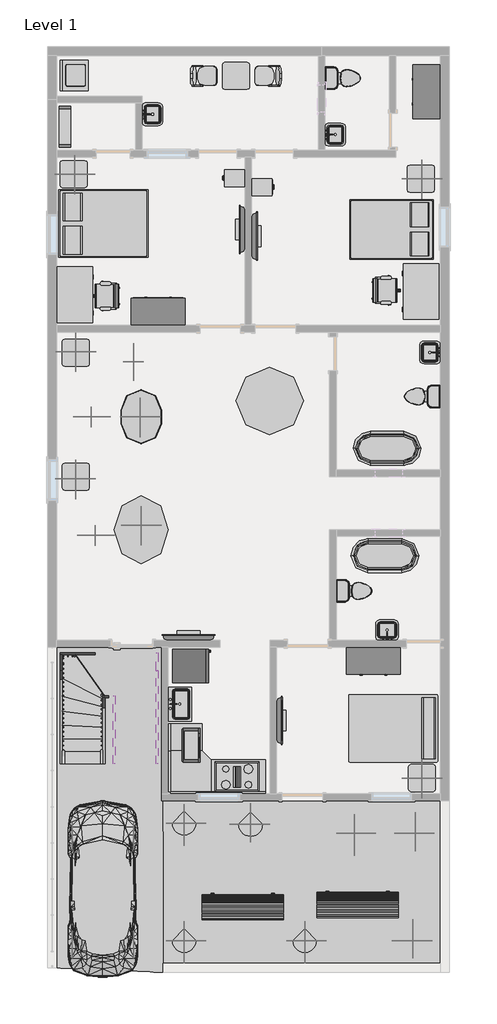
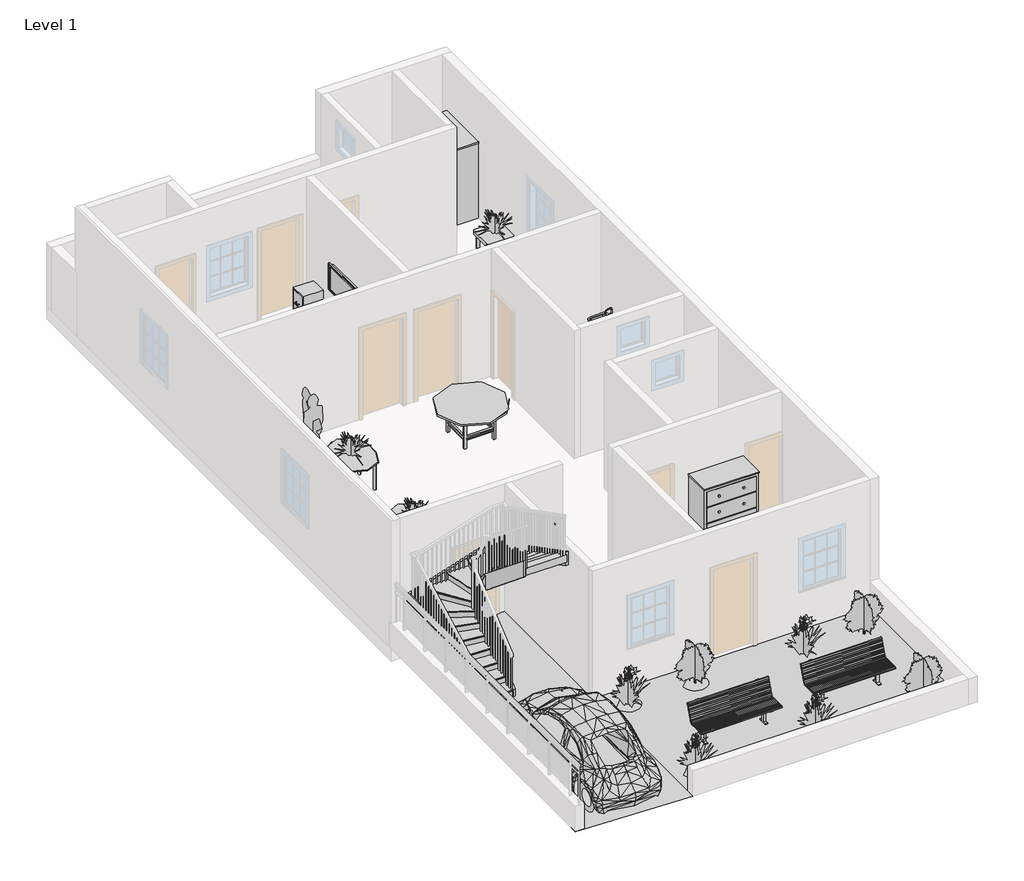
# One storey, part 3 of 3: 29 furniture elements, 16 geographic elements, 14 flow terminals, 10 proxies, 8 members, 1 stair flight.
"""IFC4 building model written with IfcOpenShell, lengths in millimetres."""

from ifc_helpers import new_model, si_unit, frame, origin, place, context, project, spatial, polyline, outline, extrude, triangles, transform, mapped, element, save
from components import proxy_bb1e6e30, proxy_8a8d5ab2, rpc_beetle_rpc_beetle_3ce7ba48, rpc_female_69e001fa, proxy_a13a33b2, proxy_718fa39f, flow_terminal_2b63360b, flow_terminal_accce45a, flow_terminal_38af2918, flow_terminal_62a433f7, toilet_domestic_3d_toilet_domestic_3d_f7549cf7, toilet_domestic_3d_toilet_domestic_3d_183bbd19, flow_terminal_b374fae2, furniture_c8abb964, furniture_1d2926bd, furniture_e1791683, furniture_bb55ed6b, chair_task_arms_chair_task_arms_fa5a08ef, furniture_8768a1f0, furniture_9fa109b2, furniture_3d1d9cbc, furniture_417d203a, furniture_7a3aaa4f, furniture_d9bcc661, furniture_be1c6672, furniture_bbcc68ce, furniture_ad1c254c, furniture_31d08a24, furniture_d6d39c5b, geographic_element_235d1464, rpc_plant_tropical_55f6ff97, rpc_plant_tropical_agave_1_5_93a2a214, rpc_plant_tropical_jungle_flame_3_9c4808c2, stair_flight_f188e120

model = new_model("IFC4")

# Units and contexts
model_context = context("Model", 3, world=origin())
ifc_project = project(units=[si_unit("LENGTHUNIT", "METRE", prefix="MILLI")], contexts=[model_context])

# Site, building, storey
site = spatial("IfcSite", under=ifc_project)
building = spatial("IfcBuilding", under=site)
storey = spatial("IfcBuildingStorey", under=building, Name="Level 1", Elevation=0.0)

# Proxies
placement = place(None, origin())
element("IfcBuildingElementProxy", 1, Name="Building Element Proxy", at=placement, inside=storey, context=model_context, shape_type="Tessellation", body=[
    triangles([(-4236.0588776, -4664.152224, 0.0), (-4236.0588776, -6188.1519333, 0.0), (-10674.9588776, -6188.1519333, 0.0), (-10713.0588776, -4664.152224, 0.0), (-10674.9588776, -8321.7519333, 0.0), (-4439.2589745, -8321.7519333, 0.0)], [[4, 5, 3], [3, 5, 6], [4, 3, 1], [2, 1, 3], [2, 3, 6]], closed=False),
])
element("IfcBuildingElementProxy", 2, Name="Building Element Proxy", at=placement, inside=storey, context=model_context, shape_type="Tessellation", body=[
    triangles([(-13075.2588776, -1209.7521755, 0.0), (-10713.0588776, -1209.7521755, 0.0), (-10674.9588776, -6188.1519333, 0.0), (-13075.2588776, -6086.5523209, 0.0), (-13167.33349, -8404.3021271, 0.0), (-10674.9588776, -8524.9523209, 0.0), (-13278.4592651, -8423.3521271, 0.0)], [[1, 7, 4], [5, 7, 6], [4, 7, 5], [3, 4, 5], [4, 2, 1], [2, 4, 3], [3, 5, 6]], closed=False),
])
proxy_shape = proxy_bb1e6e30(model_context)
element("IfcBuildingElementProxy", 3, Name="Cook Top-4 Unit : 36\" x 20\"", ObjectType="Cook Top-4 Unit : 36\" x 20\"", at=placement, inside=storey, context=model_context, shape_type="MappedRepresentation", body=[
    mapped(proxy_shape, transform((-9011.2589543, -4130.752182, 0.0), x_axis=(1.0, 0.0, 0.0), y_axis=(0.0, 1.0, 0.0), z_axis=(0.0, 0.0, 1.0))),
])
proxy_2_shape = proxy_8a8d5ab2(model_context)
element("IfcBuildingElementProxy", 4, Name="Microwave : 30\" x 16\" x 18\"", ObjectType="Microwave : 30\" x 16\" x 18\"", at=placement, inside=storey, context=model_context, shape_type="MappedRepresentation", body=[
    mapped(proxy_2_shape, transform((-10405.7394601, -3919.8450594, 0.0), x_axis=(0.0, 1.0000000000000002, 0.0), y_axis=(-1.0000000000000002, 0.0, 0.0), z_axis=(0.0, 0.0, 1.0))),
])
rpc_beetle_rpc_beetle_shape = rpc_beetle_rpc_beetle_3ce7ba48(model_context)
element("IfcBuildingElementProxy", 5, Name="RPC Beetle : RPC Beetle", ObjectType="RPC Beetle : RPC Beetle", at=placement, inside=storey, context=model_context, shape_type="MappedRepresentation", body=[
    mapped(rpc_beetle_rpc_beetle_shape, transform((-12033.8589543, -7889.952182, 0.0), x_axis=(1.0, 0.0, 0.0), y_axis=(0.0, 1.0, 0.0), z_axis=(0.0, 0.0, 1.0))),
])
rpc_female_shape = rpc_female_69e001fa(model_context)
element("IfcBuildingElementProxy", 6, Name="RPC Female", ObjectType="RPC Female", at=placement, inside=storey, context=model_context, shape_type="MappedRepresentation", body=[
    mapped(rpc_female_shape, transform((-12135.4589543, 3971.847818, 0.0), x_axis=(0.0, 1.0, 0.0), y_axis=(-1.0, 0.0, 0.0), z_axis=(0.0, 0.0, 1.0))),
])
element("IfcBuildingElementProxy", 7, Name="RPC Female", ObjectType="RPC Female", at=placement, inside=storey, context=model_context, shape_type="MappedRepresentation", body=[
    mapped(rpc_female_shape, transform((-11348.0589543, 5051.347818, 0.0), x_axis=(1.0000000000000002, 0.0, 0.0), y_axis=(0.0, 1.0000000000000002, 0.0), z_axis=(0.0, 0.0, 1.0))),
])
element("IfcBuildingElementProxy", 8, Name="RPC Female", ObjectType="RPC Female", at=placement, inside=storey, context=model_context, shape_type="MappedRepresentation", body=[
    mapped(rpc_female_shape, transform((-12046.5589543, 1304.847818, 0.0), x_axis=(0.0, 1.0000000000000002, 0.0), y_axis=(-1.0000000000000002, 0.0, 0.0), z_axis=(0.0, 0.0, 1.0))),
])
proxy_3_shape = proxy_a13a33b2(model_context)
element("IfcBuildingElementProxy", 9, Name="Refrigerator : 30\" x 32\" RH", ObjectType="Refrigerator : 30\" x 32\" RH", at=placement, inside=storey, context=model_context, shape_type="MappedRepresentation", body=[
    mapped(proxy_3_shape, transform((-10076.4714543, -1636.4011535, 0.0), x_axis=(0.0, 1.0000000000000002, 0.0), y_axis=(-1.0000000000000002, 0.0, 0.0), z_axis=(0.0, 0.0, 1.0))),
])
proxy_4_shape = proxy_718fa39f(model_context)
element("IfcBuildingElementProxy", 10, Name="Washer : 27\" x 25\" x 35\"", ObjectType="Washer : 27\" x 25\" x 35\"", at=placement, inside=storey, context=model_context, shape_type="MappedRepresentation", body=[
    mapped(proxy_4_shape, transform((-12402.4093895, 11234.9303495, 0.0), x_axis=(0.0, 1.0, 0.0), y_axis=(-1.0, 0.0, 0.0), z_axis=(0.0, 0.0, 1.0))),
])

# Flow terminals
flow_terminal_shape = flow_terminal_2b63360b(model_context)
element("IfcFlowTerminal", 11, ObjectType="Floor Drain - Rectangular : 5\"x5\" Strainer - 2\" Drain", at=placement, inside=storey, context=model_context, shape_type="MappedRepresentation", body=[
    mapped(flow_terminal_shape, transform((-5861.6589543, 11845.847818, 0.0), x_axis=(1.0, 0.0, 0.0), y_axis=(0.0, 1.0, 0.0), z_axis=(0.0, 0.0, 1.0))),
])
element("IfcFlowTerminal", 12, ObjectType="Floor Drain - Rectangular : 5\"x5\" Strainer - 2\" Drain", at=placement, inside=storey, context=model_context, shape_type="MappedRepresentation", body=[
    mapped(flow_terminal_shape, transform((-6166.4589543, 3921.047818, 0.0), x_axis=(1.0, 0.0, 0.0), y_axis=(0.0, 1.0, 0.0), z_axis=(0.0, 0.0, 1.0))),
])
element("IfcFlowTerminal", 13, ObjectType="Floor Drain - Rectangular : 5\"x5\" Strainer - 2\" Drain", at=placement, inside=storey, context=model_context, shape_type="MappedRepresentation", body=[
    mapped(flow_terminal_shape, transform((-4998.0589543, 263.447818, 0.0), x_axis=(1.0, 0.0, 0.0), y_axis=(0.0, 1.0, 0.0), z_axis=(0.0, 0.0, 1.0))),
])
flow_terminal_2_shape = flow_terminal_accce45a(model_context)
element("IfcFlowTerminal", 14, ObjectType="Floor Drain - Round : 5\" Strainer - 2\" Drain", at=placement, inside=storey, context=model_context, shape_type="MappedRepresentation", body=[
    mapped(flow_terminal_2_shape, transform((-11856.0589543, 11947.447818, 0.0), x_axis=(0.0, 1.0, 0.0), y_axis=(-1.0, 0.0, 0.0), z_axis=(0.0, 0.0, 1.0))),
])
flow_terminal_3_shape = flow_terminal_38af2918(model_context)
element("IfcFlowTerminal", 15, ObjectType="Sink Kitchen-Single : 30\" x 21\"", at=placement, inside=storey, context=model_context, shape_type="MappedRepresentation", body=[
    mapped(flow_terminal_3_shape, transform((-10304.3135531, -2508.1414226, 0.0), x_axis=(0.0, 0.9999999999999999, 0.0), y_axis=(-0.9999999999999999, 0.0, 0.0), z_axis=(0.0, 0.0, 1.0))),
])
flow_terminal_4_shape = flow_terminal_62a433f7(model_context)
element("IfcFlowTerminal", 16, ObjectType="Sink Vanity-Square : 20\" x 18\"", at=placement, inside=storey, context=model_context, shape_type="MappedRepresentation", body=[
    mapped(flow_terminal_4_shape, transform((-6849.9135531, 10306.1585774, 0.0), x_axis=(0.0, 1.0000000000000002, 0.0), y_axis=(-1.0000000000000002, 0.0, 0.0), z_axis=(0.0, 0.0, 1.0))),
])
element("IfcFlowTerminal", 17, ObjectType="Sink Vanity-Square : 20\" x 18\"", at=placement, inside=storey, context=model_context, shape_type="MappedRepresentation", body=[
    mapped(flow_terminal_4_shape, transform((-4619.4043554, 5435.3370585, 0.0), x_axis=(0.0, -1.0000000000000004, 0.0), y_axis=(1.0000000000000004, 0.0, 0.0), z_axis=(0.0, 0.0, 1.0))),
])
element("IfcFlowTerminal", 18, ObjectType="Sink Vanity-Square : 20\" x 18\"", at=placement, inside=storey, context=model_context, shape_type="MappedRepresentation", body=[
    mapped(flow_terminal_4_shape, transform((-5617.3697137, -877.2067809, 0.0), x_axis=(-1.0000000000000004, 0.0, 0.0), y_axis=(0.0, -1.0000000000000004, 0.0), z_axis=(0.0, 0.0, 1.0))),
])
element("IfcFlowTerminal", 19, ObjectType="Sink Vanity-Square : 20\" x 18\"", at=placement, inside=storey, context=model_context, shape_type="MappedRepresentation", body=[
    mapped(flow_terminal_4_shape, transform((-10964.7135531, 10763.3585774, 0.0), x_axis=(0.0, 1.0000000000000002, 0.0), y_axis=(-1.0000000000000002, 0.0, 0.0), z_axis=(0.0, 0.0, 1.0))),
])
toilet_domestic_3d_toilet_domestic_3d_shape = toilet_domestic_3d_toilet_domestic_3d_f7549cf7(model_context)
toilet_domestic_3d_toilet_domestic_3d_2_shape = toilet_domestic_3d_toilet_domestic_3d_183bbd19(model_context)
element("IfcFlowTerminal", 20, ObjectType="Toilet-Domestic-3D : Toilet-Domestic-3D", at=placement, inside=storey, context=model_context, shape_type="MappedRepresentation", body=[
    mapped(toilet_domestic_3d_toilet_domestic_3d_shape, transform((-6535.3629269, 11591.847818, 0.0), x_axis=(0.0, 1.0000000000000002, 0.0), y_axis=(-1.0000000000000002, 0.0, 0.0), z_axis=(0.0, 0.0, 1.0))),
    mapped(toilet_domestic_3d_toilet_domestic_3d_2_shape, transform((-6535.3629269, 11591.847818, 0.0), x_axis=(0.0, 1.0000000000000002, 0.0), y_axis=(-1.0000000000000002, 0.0, 0.0), z_axis=(0.0, 0.0, 1.0))),
])
element("IfcFlowTerminal", 21, ObjectType="Toilet-Domestic-3D : Toilet-Domestic-3D", at=placement, inside=storey, context=model_context, shape_type="MappedRepresentation", body=[
    mapped(toilet_domestic_3d_toilet_domestic_3d_shape, transform((-4933.9549816, 4429.047818, 0.0), x_axis=(0.0, -1.0000000000000002, 0.0), y_axis=(1.0000000000000002, 0.0, 0.0), z_axis=(0.0, 0.0, 1.0))),
    mapped(toilet_domestic_3d_toilet_domestic_3d_2_shape, transform((-4933.9549816, 4429.047818, 0.0), x_axis=(0.0, -1.0000000000000002, 0.0), y_axis=(1.0000000000000002, 0.0, 0.0), z_axis=(0.0, 0.0, 1.0))),
])
element("IfcFlowTerminal", 22, ObjectType="Toilet-Domestic-3D : Toilet-Domestic-3D", at=placement, inside=storey, context=model_context, shape_type="MappedRepresentation", body=[
    mapped(toilet_domestic_3d_toilet_domestic_3d_shape, transform((-6281.3629269, 53.4942541, 0.0), x_axis=(0.0, 1.0000000000000002, 0.0), y_axis=(-1.0000000000000002, 0.0, 0.0), z_axis=(0.0, 0.0, 1.0))),
    mapped(toilet_domestic_3d_toilet_domestic_3d_2_shape, transform((-6281.3629269, 53.4942541, 0.0), x_axis=(0.0, 1.0000000000000002, 0.0), y_axis=(-1.0000000000000002, 0.0, 0.0), z_axis=(0.0, 0.0, 1.0))),
])
flow_terminal_5_shape = flow_terminal_b374fae2(model_context)
element("IfcFlowTerminal", 23, ObjectType="Tub-Free Standing-3D : 30\" x 60\"", at=placement, inside=storey, context=model_context, shape_type="MappedRepresentation", body=[
    mapped(flow_terminal_5_shape, transform((-5633.0589543, 3260.647818, 0.0), x_axis=(0.0, 1.0000000000000002, 0.0), y_axis=(-1.0000000000000002, 0.0, 0.0), z_axis=(0.0, 0.0, 1.0))),
])
element("IfcFlowTerminal", 24, ObjectType="Tub-Free Standing-3D : 30\" x 60\"", at=placement, inside=storey, context=model_context, shape_type="MappedRepresentation", body=[
    mapped(flow_terminal_5_shape, transform((-5683.8589543, 847.647818, 0.0), x_axis=(0.0, 1.0000000000000002, 0.0), y_axis=(-1.0000000000000002, 0.0, 0.0), z_axis=(0.0, 0.0, 1.0))),
])

# Furniture
furniture_shape = furniture_c8abb964(model_context)
element("IfcFurniture", 25, ObjectType="Bed-Box : Double 53\" x 74\"", at=placement, inside=storey, context=model_context, shape_type="MappedRepresentation", body=[
    mapped(furniture_shape, transform((-5297.0294461, 8527.400277, 0.0), x_axis=(0.0, -1.0000000000000002, 0.0), y_axis=(1.0000000000000002, 0.0, 0.0), z_axis=(0.0, 0.0, 1.0))),
])
furniture_2_shape = furniture_1d2926bd(model_context)
element("IfcFurniture", 26, ObjectType="Bed-Box : Queen 60\" x 79\"", at=placement, inside=storey, context=model_context, shape_type="MappedRepresentation", body=[
    mapped(furniture_2_shape, transform((-12256.6294461, 7981.300277, 0.0), x_axis=(0.0, 1.0000000000000007, 0.0), y_axis=(-1.0000000000000007, 0.0, 0.0), z_axis=(0.0, 0.0, 1.0))),
])
furniture_3_shape = furniture_e1791683(model_context)
element("IfcFurniture", 27, ObjectType="Bed-Standard.0001 : Queen 60\" x 79\"", at=placement, inside=storey, context=model_context, shape_type="MappedRepresentation", body=[
    mapped(furniture_3_shape, transform((-5447.7638723, -2767.0636574, 0.0), x_axis=(0.0, -1.0, 0.0), y_axis=(1.0, 0.0, 0.0), z_axis=(0.0, 0.0, 1.0))),
])
furniture_4_shape = furniture_bb55ed6b(model_context)
element("IfcFurniture", 28, ObjectType="Cabinet-File 2 Drawer : 15\" x 18\"", at=placement, inside=storey, context=model_context, shape_type="MappedRepresentation", body=[
    mapped(furniture_4_shape, transform((-8919.9246541, 9216.0513709, 0.0), x_axis=(0.0, -1.0000000000000004, 0.0), y_axis=(1.0000000000000004, 0.0, 0.0), z_axis=(0.0, 0.0, 1.0))),
])
element("IfcFurniture", 29, ObjectType="Cabinet-File 2 Drawer : 15\" x 18\"", at=placement, inside=storey, context=model_context, shape_type="MappedRepresentation", body=[
    mapped(furniture_4_shape, transform((-8594.5932544, 9268.644265, 0.0), x_axis=(0.0, 1.0, 0.0), y_axis=(-1.0, 0.0, 0.0), z_axis=(0.0, 0.0, 1.0))),
])
chair_task_arms_chair_task_arms_shape = chair_task_arms_chair_task_arms_fa5a08ef(model_context)
element("IfcFurniture", 30, ObjectType="Chair-Task Arms : Chair-Task Arms", at=placement, inside=storey, context=model_context, shape_type="MappedRepresentation", body=[
    mapped(chair_task_arms_chair_task_arms_shape, transform((-11927.0540362, 6548.6569983, 0.0), x_axis=(0.0, 1.0000000000000009, 0.0), y_axis=(-1.0000000000000009, 0.0, 0.0), z_axis=(0.0, 0.0, 1.0))),
])
element("IfcFurniture", 31, ObjectType="Chair-Task Arms : Chair-Task Arms", at=placement, inside=storey, context=model_context, shape_type="MappedRepresentation", body=[
    mapped(chair_task_arms_chair_task_arms_shape, transform((-5702.8048559, 6957.6386376, 0.0), x_axis=(0.0, -1.0000000000000004, 0.0), y_axis=(1.0000000000000004, 0.0, 0.0), z_axis=(0.0, 0.0, 1.0))),
])
furniture_5_shape = furniture_8768a1f0(model_context)
element("IfcFurniture", 32, ObjectType="Desk : 60\" x 30\" Student", at=placement, inside=storey, context=model_context, shape_type="MappedRepresentation", body=[
    mapped(furniture_5_shape, transform((-13049.8589543, 7324.647818, 0.0), x_axis=(0.0, -1.0000000000000004, 0.0), y_axis=(1.0000000000000004, 0.0, 0.0), z_axis=(0.0, 0.0, 1.0))),
])
element("IfcFurniture", 33, ObjectType="Desk : 60\" x 30\" Student", at=placement, inside=storey, context=model_context, shape_type="MappedRepresentation", body=[
    mapped(furniture_5_shape, transform((-4490.0589543, 6181.647818, 0.0), x_axis=(0.0, 1.0, 0.0), y_axis=(-1.0, 0.0, 0.0), z_axis=(0.0, 0.0, 1.0))),
])
furniture_6_shape = furniture_9fa109b2(model_context)
element("IfcFurniture", 34, ObjectType="Dresser : 48\" x 72\" x 24\"", at=placement, inside=storey, context=model_context, shape_type="MappedRepresentation", body=[
    mapped(furniture_6_shape, transform((-11058.4522141, 5970.8848639, 0.0), x_axis=(-1.0000000000000004, 0.0, 0.0), y_axis=(0.0, -1.0000000000000004, 0.0), z_axis=(0.0, 0.0, 1.0))),
])
element("IfcFurniture", 35, ObjectType="Dresser : 48\" x 72\" x 24\"", at=placement, inside=storey, context=model_context, shape_type="MappedRepresentation", body=[
    mapped(furniture_6_shape, transform((-4380.8960002, 11017.8545581, 0.0), x_axis=(0.0, -1.0000000000000004, 0.0), y_axis=(1.0000000000000004, 0.0, 0.0), z_axis=(0.0, 0.0, 1.0))),
])
element("IfcFurniture", 36, ObjectType="Dresser : 48\" x 72\" x 24\"", at=placement, inside=storey, context=model_context, shape_type="MappedRepresentation", body=[
    mapped(furniture_6_shape, transform((-5668.6656944, -1151.3892279, 0.0), x_axis=(1.0, 0.0, 0.0), y_axis=(0.0, 1.0, 0.0), z_axis=(0.0, 0.0, 1.0))),
])
furniture_7_shape = furniture_3d1d9cbc(model_context)
element("IfcFurniture", 37, ObjectType="Seating-Auditorium : 18\" x 24\" x 30\"", at=placement, inside=storey, context=model_context, shape_type="MappedRepresentation", body=[
    mapped(furniture_7_shape, transform((-8110.1835444, 11481.9199491, 0.0), x_axis=(0.0, 1.0000000000000002, 0.0), y_axis=(-1.0000000000000002, 0.0, 0.0), z_axis=(0.0, 0.0, 1.0))),
])
element("IfcFurniture", 38, ObjectType="Seating-Auditorium : 18\" x 24\" x 30\"", at=placement, inside=storey, context=model_context, shape_type="MappedRepresentation", body=[
    mapped(furniture_7_shape, transform((-9963.1343641, 11803.3756868, 0.0), x_axis=(0.0, -1.0000000000000004, 0.0), y_axis=(1.0000000000000004, 0.0, 0.0), z_axis=(0.0, 0.0, 1.0))),
])
furniture_8_shape = furniture_417d203a(model_context)
element("IfcFurniture", 39, ObjectType="Shelving : 36\" x 10\" x 72\"", at=placement, inside=storey, context=model_context, shape_type="MappedRepresentation", body=[
    mapped(furniture_8_shape, transform((-13195.9089543, 10499.647818, 0.0), x_axis=(0.0, 1.0000000000000002, 0.0), y_axis=(-1.0000000000000002, 0.0, 0.0), z_axis=(0.0, 0.0, 1.0))),
])
furniture_9_shape = furniture_7a3aaa4f(model_context)
element("IfcFurniture", 40, ObjectType="TV - Flat Screen : 42\"", at=placement, inside=storey, context=model_context, shape_type="MappedRepresentation", body=[
    mapped(furniture_9_shape, transform((-8891.9975779, 8184.3033038, 990.6), x_axis=(0.0, -1.0000000000000004, 0.0), y_axis=(1.0000000000000004, 0.0, 0.0), z_axis=(0.0, 0.0, 1.0))),
])
element("IfcFurniture", 41, ObjectType="TV - Flat Screen : 42\"", at=placement, inside=storey, context=model_context, shape_type="MappedRepresentation", body=[
    mapped(furniture_9_shape, transform((-8622.5203306, 8039.7923321, 1041.4), x_axis=(0.0, 1.0000000000000002, 0.0), y_axis=(-1.0000000000000002, 0.0, 0.0), z_axis=(0.0, 0.0, 1.0))),
])
element("IfcFurniture", 42, ObjectType="TV - Flat Screen : 42\"", at=placement, inside=storey, context=model_context, shape_type="MappedRepresentation", body=[
    mapped(furniture_9_shape, transform((-8063.7203306, -2856.8076679, 990.6), x_axis=(0.0, 1.0000000000000002, 0.0), y_axis=(-1.0000000000000002, 0.0, 0.0), z_axis=(0.0, 0.0, 1.0))),
])
furniture_10_shape = furniture_d9bcc661(model_context)
element("IfcFurniture", 43, ObjectType="TV - Flat Screen : 46\"", at=placement, inside=storey, context=model_context, shape_type="MappedRepresentation", body=[
    mapped(furniture_10_shape, transform((-10107.4034684, -998.8135584, 990.6), x_axis=(-1.0000000000000004, 0.0, 0.0), y_axis=(0.0, -1.0000000000000004, 0.0), z_axis=(0.0, 0.0, 1.0))),
])
furniture_11_shape = furniture_be1c6672(model_context)
element("IfcFurniture", 44, ObjectType="Table-Dining Oval : 36\" x 48\"", at=placement, inside=storey, context=model_context, shape_type="MappedRepresentation", body=[
    mapped(furniture_11_shape, transform((-11528.3573149, 4373.6674901, 0.0), x_axis=(0.0, 1.0000000000000002, 0.0), y_axis=(-1.0000000000000002, 0.0, 0.0), z_axis=(0.0, 0.0, 1.0))),
])
furniture_12_shape = furniture_bbcc68ce(model_context)
element("IfcFurniture", 45, ObjectType="Table-Dining Round w Chairs : 60\" Diameter", at=placement, inside=storey, context=model_context, shape_type="MappedRepresentation", body=[
    mapped(furniture_12_shape, transform((-8380.3934379, 4513.303937, 0.0), x_axis=(1.0, 0.0, 0.0), y_axis=(0.0, 1.0, 0.0), z_axis=(0.0, 0.0, 1.0))),
])
furniture_13_shape = furniture_ad1c254c(model_context)
element("IfcFurniture", 46, ObjectType="Table-Ellipse : 60\" x 48\"", at=placement, inside=storey, context=model_context, shape_type="MappedRepresentation", body=[
    mapped(furniture_13_shape, transform((-11170.2589543, 1431.847818, 0.0), x_axis=(0.0, 1.0, 0.0), y_axis=(-1.0, 0.0, 0.0), z_axis=(0.0, 0.0, 1.0))),
])
furniture_14_shape = furniture_31d08a24(model_context)
element("IfcFurniture", 47, ObjectType="Table-End : 24\" x 24\"", at=placement, inside=storey, context=model_context, shape_type="MappedRepresentation", body=[
    mapped(furniture_14_shape, transform((-13002.7925845, 9280.447818, 0.0), x_axis=(1.0, 0.0, 0.0), y_axis=(0.0, 1.0, 0.0), z_axis=(0.0, 0.0, 1.0))),
])
element("IfcFurniture", 48, ObjectType="Table-End : 24\" x 24\"", at=placement, inside=storey, context=model_context, shape_type="MappedRepresentation", body=[
    mapped(furniture_14_shape, transform((-9345.1925845, 11490.247818, 0.0), x_axis=(1.0, 0.0, 0.0), y_axis=(0.0, 1.0, 0.0), z_axis=(0.0, 0.0, 1.0))),
])
element("IfcFurniture", 49, ObjectType="Table-End : 24\" x 24\"", at=placement, inside=storey, context=model_context, shape_type="MappedRepresentation", body=[
    mapped(furniture_14_shape, transform((-5179.5925845, 9178.847818, 0.0), x_axis=(1.0, 0.0, 0.0), y_axis=(0.0, 1.0, 0.0), z_axis=(0.0, 0.0, 1.0))),
])
element("IfcFurniture", 50, ObjectType="Table-End : 24\" x 24\"", at=placement, inside=storey, context=model_context, shape_type="MappedRepresentation", body=[
    mapped(furniture_14_shape, transform((-5154.1925845, -4308.552182, 0.0), x_axis=(1.0, 0.0, 0.0), y_axis=(0.0, 1.0, 0.0), z_axis=(0.0, 0.0, 1.0))),
])
element("IfcFurniture", 51, ObjectType="Table-End : 24\" x 24\"", at=placement, inside=storey, context=model_context, shape_type="MappedRepresentation", body=[
    mapped(furniture_14_shape, transform((-12951.9925845, 5260.897818, 0.0), x_axis=(1.0, 0.0, 0.0), y_axis=(0.0, 1.0, 0.0), z_axis=(0.0, 0.0, 1.0))),
])
element("IfcFurniture", 52, ObjectType="Table-End : 24\" x 24\"", at=placement, inside=storey, context=model_context, shape_type="MappedRepresentation", body=[
    mapped(furniture_14_shape, transform((-12951.9925845, 2473.247818, 0.0), x_axis=(1.0, 0.0, 0.0), y_axis=(0.0, 1.0, 0.0), z_axis=(0.0, 0.0, 1.0))),
])
furniture_15_shape = furniture_d6d39c5b(model_context)
element("IfcFurniture", 53, ObjectType="Work Station Cubicle : 96\" x 96\"", at=placement, inside=storey, context=model_context, shape_type="MappedRepresentation", body=[
    mapped(furniture_15_shape, transform((-11055.6819619, -4380.0204298, 0.0), x_axis=(0.0, 1.0, 0.0), y_axis=(-1.0, 0.0, 0.0), z_axis=(0.0, 0.0, 1.0))),
])

# Geographic elements
geographic_element_shape = geographic_element_235d1464(model_context)
element("IfcGeographicElement", 54, ObjectType="Park Bench : 72\"", at=placement, inside=storey, context=model_context, shape_type="MappedRepresentation", body=[
    mapped(geographic_element_shape, transform((-8884.2589543, -7026.352182, 0.0), x_axis=(1.0, 0.0, 0.0), y_axis=(0.0, 1.0, 0.0), z_axis=(0.0, 0.0, 1.0))),
])
element("IfcGeographicElement", 55, ObjectType="Park Bench : 72\"", at=placement, inside=storey, context=model_context, shape_type="MappedRepresentation", body=[
    mapped(geographic_element_shape, transform((-6293.4589543, -6975.552182, 0.0), x_axis=(1.0, 0.0, 0.0), y_axis=(0.0, 1.0, 0.0), z_axis=(0.0, 0.0, 1.0))),
])
rpc_plant_tropical_shape = rpc_plant_tropical_55f6ff97(model_context)
element("IfcGeographicElement", 56, ObjectType="RPC Plant - Tropical", at=placement, inside=storey, context=model_context, shape_type="MappedRepresentation", body=[
    mapped(rpc_plant_tropical_shape, transform((-6369.6589543, -5400.752182, 0.0), x_axis=(1.0, 0.0, 0.0), y_axis=(0.0, 1.0, 0.0), z_axis=(0.0, 0.0, 1.0))),
])
element("IfcGeographicElement", 57, ObjectType="RPC Plant - Tropical", at=placement, inside=storey, context=model_context, shape_type="MappedRepresentation", body=[
    mapped(rpc_plant_tropical_shape, transform((-10205.0589543, -5172.152182, 0.0), x_axis=(1.0, 0.0, 0.0), y_axis=(0.0, 1.0, 0.0), z_axis=(0.0, 0.0, 1.0))),
])
element("IfcGeographicElement", 58, ObjectType="RPC Plant - Tropical", at=placement, inside=storey, context=model_context, shape_type="MappedRepresentation", body=[
    mapped(rpc_plant_tropical_shape, transform((-7487.2589543, -7813.752182, 0.0), x_axis=(1.0, 0.0, 0.0), y_axis=(0.0, 1.0, 0.0), z_axis=(0.0, 0.0, 1.0))),
])
element("IfcGeographicElement", 59, ObjectType="RPC Plant - Tropical", at=placement, inside=storey, context=model_context, shape_type="MappedRepresentation", body=[
    mapped(rpc_plant_tropical_shape, transform((-10205.0589543, -7813.752182, 0.0), x_axis=(1.0, 0.0, 0.0), y_axis=(0.0, 1.0, 0.0), z_axis=(0.0, 0.0, 1.0))),
])
rpc_plant_tropical_agave_1_5_shape = rpc_plant_tropical_agave_1_5_93a2a214(model_context)
element("IfcGeographicElement", 60, ObjectType="RPC Plant - Tropical : Agave - 1.5'", at=placement, inside=storey, context=model_context, shape_type="MappedRepresentation", body=[
    mapped(rpc_plant_tropical_agave_1_5_shape, transform((-12668.8589543, 9432.847818, 609.6), x_axis=(1.0, 0.0, 0.0), y_axis=(0.0, 1.0, 0.0), z_axis=(0.0, 0.0, 1.0))),
])
element("IfcGeographicElement", 61, ObjectType="RPC Plant - Tropical : Agave - 1.5'", at=placement, inside=storey, context=model_context, shape_type="MappedRepresentation", body=[
    mapped(rpc_plant_tropical_agave_1_5_shape, transform((-4845.6589543, 9331.247818, 609.6), x_axis=(1.0, 0.0, 0.0), y_axis=(0.0, 1.0, 0.0), z_axis=(0.0, 0.0, 1.0))),
])
element("IfcGeographicElement", 62, ObjectType="RPC Plant - Tropical : Agave - 1.5'", at=placement, inside=storey, context=model_context, shape_type="MappedRepresentation", body=[
    mapped(rpc_plant_tropical_agave_1_5_shape, transform((-4845.6589543, -4156.152182, 609.6), x_axis=(1.0, 0.0, 0.0), y_axis=(0.0, 1.0, 0.0), z_axis=(0.0, 0.0, 1.0))),
])
element("IfcGeographicElement", 63, ObjectType="RPC Plant - Tropical : Agave - 1.5'", at=placement, inside=storey, context=model_context, shape_type="MappedRepresentation", body=[
    mapped(rpc_plant_tropical_agave_1_5_shape, transform((-11195.6589543, 3971.847818, 762.0), x_axis=(1.0, 0.0, 0.0), y_axis=(0.0, 1.0, 0.0), z_axis=(0.0, 0.0, 1.0))),
])
element("IfcGeographicElement", 64, ObjectType="RPC Plant - Tropical : Agave - 1.5'", at=placement, inside=storey, context=model_context, shape_type="MappedRepresentation", body=[
    mapped(rpc_plant_tropical_agave_1_5_shape, transform((-11170.2589543, 1533.447818, 660.4), x_axis=(1.0, 0.0, 0.0), y_axis=(0.0, 1.0, 0.0), z_axis=(0.0, 0.0, 1.0))),
])
element("IfcGeographicElement", 65, ObjectType="RPC Plant - Tropical : Agave - 1.5'", at=placement, inside=storey, context=model_context, shape_type="MappedRepresentation", body=[
    mapped(rpc_plant_tropical_agave_1_5_shape, transform((-12643.4589543, 5438.697818, 609.6), x_axis=(1.0, 0.0, 0.0), y_axis=(0.0, 1.0, 0.0), z_axis=(0.0, 0.0, 1.0))),
])
element("IfcGeographicElement", 66, ObjectType="RPC Plant - Tropical : Agave - 1.5'", at=placement, inside=storey, context=model_context, shape_type="MappedRepresentation", body=[
    mapped(rpc_plant_tropical_agave_1_5_shape, transform((-12649.8089543, 2574.847818, 609.6), x_axis=(1.0, 0.0, 0.0), y_axis=(0.0, 1.0, 0.0), z_axis=(0.0, 0.0, 1.0))),
])
rpc_plant_tropical_jungle_flame_3_shape = rpc_plant_tropical_jungle_flame_3_9c4808c2(model_context)
element("IfcGeographicElement", 67, ObjectType="RPC Plant - Tropical : Jungle Flame - 3'", at=placement, inside=storey, context=model_context, shape_type="MappedRepresentation", body=[
    mapped(rpc_plant_tropical_jungle_flame_3_shape, transform((-4998.0589543, -5400.752182, 0.0), x_axis=(1.0, 0.0, 0.0), y_axis=(0.0, 1.0, 0.0), z_axis=(0.0, 0.0, 1.0))),
])
element("IfcGeographicElement", 68, ObjectType="RPC Plant - Tropical : Jungle Flame - 3'", at=placement, inside=storey, context=model_context, shape_type="MappedRepresentation", body=[
    mapped(rpc_plant_tropical_jungle_flame_3_shape, transform((-8706.4589543, -5197.552182, 0.0), x_axis=(1.0, 0.0, 0.0), y_axis=(0.0, 1.0, 0.0), z_axis=(0.0, 0.0, 1.0))),
])
element("IfcGeographicElement", 69, ObjectType="RPC Plant - Tropical : Jungle Flame - 3'", at=placement, inside=storey, context=model_context, shape_type="MappedRepresentation", body=[
    mapped(rpc_plant_tropical_jungle_flame_3_shape, transform((-5048.8589543, -7813.752182, 0.0), x_axis=(1.0, 0.0, 0.0), y_axis=(0.0, 1.0, 0.0), z_axis=(0.0, 0.0, 1.0))),
])

# Members
element("IfcMember", 70, ObjectType="Stringer - 2\" Width", at=placement, inside=storey, context=model_context, shape_type="SweptSolid", body=[
    extrude(outline(polyline([(-3829.6838739, 0.0), (-3829.6838739, 229.639954), (-1742.2666822, 1305.3956453), (-1742.2666822, 962.500629), (-3609.9215563, 0.0), (-3829.6838739, 0.0)])), frame((-12999.0589543, 0.0, 0.0), z_axis=(1.0, 0.0, 0.0), x_axis=(0.0, 1.0, 0.0)), (0.0, 0.0, 1.0), 50.8),
])
element("IfcMember", 71, ObjectType="Stringer - 2\" Width", at=placement, inside=storey, context=model_context, shape_type="SweptSolid", body=[
    extrude(outline(polyline([(-12948.2589543, -1742.2666822), (-12999.0589543, -1742.2666822), (-12999.0589543, -1387.552182), (-12948.2589543, -1387.552182), (-12948.2589543, -1742.2666822)])), frame((0.0, 0.0, 962.500629), z_axis=(0.0, 0.0, 1.0), x_axis=(1.0, 0.0, 0.0)), (0.0, 0.0, 1.0), 342.8950162),
])
element("IfcMember", 72, ObjectType="Stringer - 2\" Width", at=placement, inside=storey, context=model_context, shape_type="SweptSolid", body=[
    extrude(outline(polyline([(1289.0952212, -12999.0589543), (1000.5956453, -12999.0589543), (1000.5956453, -12829.5364713), (1638.9682298, -10840.0589543), (1969.9972697, -10840.0589543), (1969.9972697, -10877.0390715), (1289.0952212, -12999.0589543)])), frame((0.0, -1387.552182, 0.0), z_axis=(0.0, 1.0, 0.0), x_axis=(0.0, 0.0, 1.0)), (0.0, 0.0, 1.0), 50.8),
])
element("IfcMember", 73, ObjectType="Stringer - 2\" Width", at=placement, inside=storey, context=model_context, shape_type="SweptSolid", body=[
    extrude(outline(polyline([(-10840.0589543, -1336.752182), (-10789.2589543, -1336.752182), (-10789.2589543, -1742.2666822), (-10840.0589543, -1742.2666822), (-10840.0589543, -1336.752182)])), frame((0.0, 0.0, 1649.8904473), z_axis=(0.0, 0.0, 1.0), x_axis=(1.0, 0.0, 0.0)), (0.0, 0.0, 1.0), 320.1068224),
])
element("IfcMember", 74, ObjectType="Stringer - 2\" Width", at=placement, inside=storey, context=model_context, shape_type="SweptSolid", body=[
    extrude(outline(polyline([(-1742.2666822, 1969.9972697), (-1742.2666822, 1649.8904473), (-3829.6838739, 2725.6461385), (-3829.6838739, 3045.7529609), (-1742.2666822, 1969.9972697)])), frame((-10840.0589543, 0.0, 0.0), z_axis=(1.0, 0.0, 0.0), x_axis=(0.0, 1.0, 0.0)), (0.0, 0.0, 1.0), 50.8),
])
element("IfcMember", 75, ObjectType="Stringer - 2\" Width", at=placement, inside=storey, context=model_context, shape_type="SweptSolid", body=[
    extrude(outline(polyline([(-3829.6838739, 0.0), (-3829.6838739, 176.1764461), (-2352.752182, 1380.418648), (-2352.752182, 987.1410923), (-3563.4222293, 0.0), (-3829.6838739, 0.0)])), frame((-12033.8589543, 0.0, 0.0), z_axis=(1.0, 0.0, 0.0), x_axis=(0.0, 1.0, 0.0)), (0.0, 0.0, 1.0), 50.8),
])
element("IfcMember", 76, ObjectType="Stringer - 2\" Width", at=placement, inside=storey, context=model_context, shape_type="SweptSolid", body=[
    extrude(outline(polyline([(1573.2682978, -12033.8589543), (1028.5617647, -12033.8589543), (1028.5617647, -11999.6167369), (1360.465107, -11805.2589543), (1926.1409689, -11805.2589543), (1926.1409689, -11827.2218368), (1573.2682978, -12033.8589543)])), frame((0.0, -2352.752182, 0.0), z_axis=(0.0, 1.0, 0.0), x_axis=(0.0, 0.0, 1.0)), (0.0, 0.0, 1.0), 50.8),
])
element("IfcMember", 77, ObjectType="Stringer - 2\" Width", at=placement, inside=storey, context=model_context, shape_type="SweptSolid", body=[
    extrude(outline(polyline([(-2301.952182, 1926.1409689), (-2301.952182, 1532.8634131), (-3829.6838739, 2778.5262875), (-3829.6838739, 3171.8038432), (-2301.952182, 1926.1409689)])), frame((-11805.2589543, 0.0, 0.0), z_axis=(1.0, 0.0, 0.0), x_axis=(0.0, 1.0, 0.0)), (0.0, 0.0, 1.0), 50.8),
])

# Stair flight
stair_flight_shape = stair_flight_f188e120(model_context)
element("IfcStairFlight", 78, ObjectType="2\" Tread 1\" Nosing 1/4\" Riser", at=placement, inside=storey, context=model_context, shape_type="MappedRepresentation", body=[
    mapped(stair_flight_shape, transform((0.0, 0.0, 0.0), x_axis=(1.0, 0.0, 0.0), y_axis=(0.0, 1.0, 0.0), z_axis=(0.0, 0.0, 1.0))),
])

save(model, "model.ifc")

# Revit data of these elements
# Type "Cook Top-4 Unit : 36\" x 20\""
#   Assembly Code = "E1090400"
#   Depth = 2' - 0"
#   Width = 3' - 0"
#   Burner Material = Steel, Chrome Plated
#   Cooktop Material = Steel, Polished
#   Default Elevation = 0
# Type "Microwave : 30\" x 16\" x 18\""
#   Assembly Code = "E1090400"
#   Depth = 1' - 4"
#   Height = 1' - 6"
#   Width = 2' - 6"
#   Microwave Material = Laminate - Ivory, Glossy
#   Default Elevation = 0
# Type "RPC Beetle : RPC Beetle"
#   built-in parameter 1005195 = "RPC-16-0U6E-L4EG-ENH1-J3KF-SVEL-0TX4-C0"
#   Height = 0
# Type "RPC Female"
#   built-in parameter 1005195 = "RPC-8-FXA2-QQQ0-UGV2-6"
#   Height = 0
# Type "Refrigerator : 30\" x 32\" RH"
#   Label = "REF."
#   Assembly Code = "E1090400"
#   Depth = 2' - 7 3/4"
#   Handle = 2' - 3"
#   Height = 5' - 10"
#   Rear Clearance = 0' - 2"
#   Top Door Height = 1' - 8"
#   Width = 2' - 5 3/8"
#   Material = Steel, Paint Finish, Ivory, Glossy
#   Default Elevation = 0
# Type "Washer : 27\" x 25\" x 35\""
#   Label = "W"
#   Assembly Code = "E1090400"
#   Depth = 2' - 1"
#   Height = 2' - 11"
#   Width = 2' - 3"
#   Washer Material = Steel, Paint Finish, Ivory, Matte
#   Default Elevation = 0
# Type "Floor Drain - Rectangular : 5\"x5\" Strainer - 2\" Drain"
#   WFU = 2
#   Strainer Height = 0' - 3 1/4"
#   Half Strainer Length = 0' - 2 1/2"
#   Strainer Length = 0' - 5"
#   Radius 2 = 0' - 3.04167"
#   Radius 1 = 0' - 2.02083"
#   Radius 3 = 0' - 2 1/32"
#   Pipe Radius = 1"
#   Pipe Diameter = 2"
#   Height 2 = 0' - 0.725"
#   Height 1 = 0' - 1 13/16"
#   Body Radius = 0' - 4 1/16"
#   Body Height = 0' - 3 5/8"
#   Body Diameter = 0' - 8 1/8"
#   Drain Material = none
#   HWFU = 0
#   Default Elevation = 0
#   CWFU = 0
# Type "Floor Drain - Round : 5\" Strainer - 2\" Drain"
#   WFU = 2
#   Strainer Height = 0' - 3 1/4"
#   Strainer Radius = 0' - 2 1/2"
#   Strainer Diameter = 0' - 5"
#   Radius 6 = 0' - 0 5/8"
#   Radius 5 = 0' - 1 1/4"
#   Radius 4 = 0' - 1 7/8"
#   Radius 2 = 0' - 3.04167"
#   Radius 1 = 0' - 2.02083"
#   Radius 3 = 0' - 2 1/32"
#   Pipe Radius = 1"
#   Pipe Diameter = 2"
#   Height 2 = 0' - 0.725"
#   Height 1 = 0' - 1 13/16"
#   Body Radius = 0' - 4 1/16"
#   Body Height = 0' - 3 5/8"
#   Body Diameter = 0' - 8 1/8"
#   Drain Material = none
#   HWFU = 0
#   Default Elevation = 0
#   CWFU = 0
# Type "Sink Kitchen-Single : 30\" x 21\""
#   Assembly Code = "D2010410"
#   Counter Height = 3' - 0"
#   Depth = 1' - 9"
#   Width = 2' - 6"
#   Faucet Material = Steel, Polished
#   Sink Material = Steel, Polished
#   Default Elevation = 0
# Type "Sink Vanity-Square : 20\" x 18\""
#   Assembly Code = "D2010400"
#   Counter Height = 2' - 7"
#   Depth = 1' - 6"
#   Width = 1' - 8"
#   Basin Material = Porcelain, Linen
#   Faucet Material = Steel, Polished
#   Default Elevation = 0
# Type "Toilet-Domestic-3D : Toilet-Domestic-3D"
#   Assembly Code = "D2010110"
#   Toilet - Bowl/Basin Material = Porcelain, Linen
#   Toilet - Seat Material = Laminate, Linen, Matte
#   Default Elevation = 0
# Type "Tub-Free Standing-3D : 30\" x 60\""
#   Assembly Code = "D2010110"
#   Height = 1' - 6"
#   Length = 5' - 0"
#   Width = 2' - 6"
#   Tub Material = Porcelain, Ivory
#   Default Elevation = 0
# Type "Bed-Box : Double 53\" x 74\""
#   Assembly Code = "E2020200"
#   Length = 6' - 2"
#   Width = 4' - 5"
#   Frame Material = Birch
#   Mattress Material = Sash
#   Default Elevation = 0
# Type "Bed-Box : Queen 60\" x 79\""
#   Assembly Code = "E2020200"
#   Length = 6' - 7"
#   Width = 5' - 0"
#   Frame Material = Birch
#   Mattress Material = Sash
#   Default Elevation = 0
# Type "Bed-Standard.0001 : Queen 60\" x 79\""
#   Assembly Code = "E2020200"
#   Length = 6' - 7"
#   Width = 5' - 0"
#   Leg Material = Steel, Chrome Plated
#   Mattress Material = Sash
#   Default Elevation = 0
# Type "Cabinet-File 2 Drawer : 15\" x 18\""
#   Assembly Code = "E2020200"
#   Depth = 1' - 6"
#   Height = 2' - 5"
#   Width = 1' - 3"
#   Cabinet Material = Steel, Paint Finish, Ivory, Glossy
#   Handle Material = Steel, Chrome Plated
#   Default Elevation = 0
# Type "Chair-Task Arms : Chair-Task Arms"
#   Assembly Code = "E2020200"
#   Base Material = Plastic, Opaque Black
#   Caster Material = Plastic, Opaque Black
#   Seat/Back Material = Textile - Slate Blue
#   Default Elevation = 0
# Type "Desk : 60\" x 30\" Student"
#   Assembly Code = "E2020200"
#   Depth = 2' - 6"
#   Height = 2' - 6"
#   Leg Height = 0' - 6"
#   Width = 4' - 0"
#   Body Material = Laminate, Ivory, Matte
#   Handle/Leg Material = Steel, Chrome Plated
#   Top Material = Cherry
#   Default Elevation = 0
# Type "Dresser : 48\" x 72\" x 24\""
#   Assembly Code = "E2020200"
#   Depth = 2' - 0"
#   Height = 6' - 0"
#   Width = 4' - 0"
#   Dresser Material = Wood - Teak
#   Drawer Material = Wood - Teak
#   Knob Material = Cherry
#   Default Elevation = 0
# Type "Seating-Auditorium : 18\" x 24\" x 30\""
#   Assembly Code = "E2020200"
#   Seat Material = Linen, Beige
#   Frame Material = Steel, Paint Finish, Dark Gray, Matte
#   Default Elevation = 0
# Type "Shelving : 36\" x 10\" x 72\""
#   Assembly Code = "E2020200"
#   Depth = 0' - 10"
#   Height = 6' - 0"
#   Width = 3' - 0"
#   Shelving Unit Material = Birch
#   Default Elevation = 0
# Type "TV - Flat Screen : 42\""
#   SinAng = 0' - 0.0193"
#   L = 3' - 0.71517"
#   H = 1' - 8.65418"
#   Thickness = 0' - 4.33071"
#   Diagonal = 3' - 6.12598"
#   CosAng = 0' - 0.03431"
#   Stand [instance default] = yes
#   Default Elevation = 0
# Type "TV - Flat Screen : 46\""
#   SinAng = 0' - 0.0193"
#   L = 3' - 4.83276"
#   H = 1' - 10.97053"
#   Thickness = 0' - 4.33071"
#   Diagonal = 3' - 10.85039"
#   CosAng = 0' - 0.03431"
#   Stand [instance default] = yes
#   Default Elevation = 0
# Type "Table-Dining Oval : 36\" x 48\""
#   Assembly Code = "E2020200"
#   Length = 4' - 0"
#   Width = 3' - 0"
#   Base Material = Steel, Chrome Plated
#   Top Material = Glass - Clear, Grey
#   Default Elevation = 0
#   Description = (empty or 0)
# Type "Table-Dining Round w Chairs : 60\" Diameter"
#   Assembly Code = "E2020200"
#   Radius = 2' - 6"
#   Diameter = 5' - 0"
#   Height = 2' - 6"
#   Chairs = 6
#   Base Material = Pine
#   Top Material = Laminate, Linen, Matte
#   Default Elevation = 0
# Type "Table-Ellipse : 60\" x 48\""
#   Assembly Code = "E2020200"
#   Half Width = 2' - 0"
#   Half Length = 2' - 6"
#   Height = 2' - 2"
#   Length = 5' - 0"
#   Width = 4' - 0"
#   Base Material = Birch
#   Top Material = Birch
#   Default Elevation = 0
# Type "Table-End : 24\" x 24\""
#   Assembly Code = "E2020200"
#   Height = 2' - 0"
#   Length = 2' - 0"
#   Width = 2' - 0"
#   Base Material = Birch
#   Top Material = Laminate, Ivory, Matte
#   Default Elevation = 0
# Type "Work Station Cubicle : 96\" x 96\""
#   Assembly Code = "E2020"
#   Desktop Height = 2' - 6"
#   Desktop1 Width = 2' - 4"
#   Desktop2 Width = 2' - 4"
#   Panel Height = 2' - 8"
#   Panel1 Length = 4' - 0"
#   Panel2 Length = 2' - 0"
#   Cube Panel Material = Textile - Light Gray
#   Work Top Material = Laminate, Ivory, Matte
#   Default Elevation = 0
# Type "Park Bench : 72\""
#   Length = 6' - 0"
#   Seat Material = Wood - Teak
#   Frame Material = Steel, Paint Finish, Dark Gray, Matte
# Type "RPC Plant - Tropical"
#   built-in parameter 1005198 = "{2, 15},{39, RPC-16-FWM5-GM7X-C67P-4000-ST1L-LVER-AU},{1, 0},{1, 0},{2, 13},{1, 8},{5, Color},{1, 0},{1, 0},{3, 0.8},{3, 0.8},{3, 0.8},{1, 8},{7, BBoxMin},{1, 0},{1, 0},{1, 0},{1, 0},{1, 0},{1, 8},{7, BBoxMax},{1, 0},{1, 0},{1, 0},{1, 0},{1, 0},{2, 11},{9, RPCTypeId},{1, 0},{1, 0},{39, RPC-16-FWM5-GM7X-C67P-4000-ST1L-LVER-AU},{1, 6},{14, RPCPlantHeight},{1, 0},{1, 0},{1, 3},{2, 11},{7, keyword},{1, 0},{1, 0},{35, :RPCs:Shrubs [General]:Geometry:RPC},{2, 11},{8, category},{1, 0},{1, 0},{16, Shrubs [General]},{2, 11},{12, LocalizedUID},{1, 0},{1, 0},{10, Crane Lily},{2, 14},{6, Height},{1, 0},{1, 0},{1, 3},{1, 2},{16, Cast Reflections},{1, 0},{1, 0},{1, 0},{1, 2},{12, Cast Shadows},{1, 0},{1, 0},{1, 1},{1, 2},{9, Lock View},{1, 0},{1, 0},{1, 0},{1, 4},{5, ViewC},{1, 0},{1, 0},{1, 0},{21, assetlibrary_base.fbx},{1, 5},"
#   built-in parameter 1005195 = "RPC-16-FWM5-GM7X-C67P-4000-ST1L-LVER-AU"
#   Assembly Code = "G2050500"
#   Height = 3' - 0"
#   Default Elevation = 0
# Type "RPC Plant - Tropical : Agave - 1.5'"
#   built-in parameter 1005198 = "{2, 15},{39, RPC-16-G1GJ-63FX-7K5P-N000-ST1L-LVER-AU},{1, 0},{1, 0},{2, 13},{1, 8},{5, Color},{1, 0},{1, 0},{3, 0.8},{3, 0.8},{3, 0.8},{1, 8},{7, BBoxMin},{1, 0},{1, 0},{1, 0},{1, 0},{1, 0},{1, 8},{7, BBoxMax},{1, 0},{1, 0},{1, 0},{1, 0},{1, 0},{2, 11},{9, RPCTypeId},{1, 0},{1, 0},{39, RPC-16-G1GJ-63FX-7K5P-N000-ST1L-LVER-AU},{1, 6},{14, RPCPlantHeight},{1, 0},{1, 0},{3, 1.5},{2, 11},{7, keyword},{1, 0},{1, 0},{35, :RPCs:Plants [General]:Geometry:RPC},{2, 11},{8, category},{1, 0},{1, 0},{16, Plants [General]},{2, 11},{12, LocalizedUID},{1, 0},{1, 0},{5, Agave},{2, 14},{6, Height},{1, 0},{1, 0},{3, 1.5},{1, 2},{16, Cast Reflections},{1, 0},{1, 0},{1, 0},{1, 2},{12, Cast Shadows},{1, 0},{1, 0},{1, 1},{1, 2},{9, Lock View},{1, 0},{1, 0},{1, 0},{1, 4},{5, ViewC},{1, 0},{1, 0},{1, 0},{21, assetlibrary_base.fbx},{1, 5},"
#   built-in parameter 1005195 = "RPC-16-G1GJ-63FX-7K5P-N000-ST1L-LVER-AU"
#   Type Comments = "Agave"
#   Assembly Code = "G2050500"
#   Height = 1' - 6"
#   Default Elevation = 0
# Type "RPC Plant - Tropical : Jungle Flame - 3'"
#   built-in parameter 1005198 = "{2, 15},{39, RPC-16-FUVJ-JWG0-MWGK-8000-ST1L-LVER-AU},{1, 0},{1, 0},{2, 13},{1, 8},{5, Color},{1, 0},{1, 0},{3, 0.8},{3, 0.8},{3, 0.8},{1, 8},{7, BBoxMin},{1, 0},{1, 0},{1, 0},{1, 0},{1, 0},{1, 8},{7, BBoxMax},{1, 0},{1, 0},{1, 0},{1, 0},{1, 0},{2, 11},{9, RPCTypeId},{1, 0},{1, 0},{39, RPC-16-FUVJ-JWG0-MWGK-8000-ST1L-LVER-AU},{1, 6},{14, RPCPlantHeight},{1, 0},{1, 0},{1, 3},{2, 11},{7, keyword},{1, 0},{1, 0},{35, :RPCs:Shrubs [General]:Geometry:RPC},{2, 11},{8, category},{1, 0},{1, 0},{16, Shrubs [General]},{2, 11},{12, LocalizedUID},{1, 0},{1, 0},{12, Jungle Flame},{2, 14},{6, Height},{1, 0},{1, 0},{1, 3},{1, 2},{16, Cast Reflections},{1, 0},{1, 0},{1, 0},{1, 2},{12, Cast Shadows},{1, 0},{1, 0},{1, 1},{1, 2},{9, Lock View},{1, 0},{1, 0},{1, 0},{1, 4},{5, ViewC},{1, 0},{1, 0},{1, 0},{21, assetlibrary_base.fbx},{1, 5},"
#   built-in parameter 1005195 = "RPC-16-FUVJ-JWG0-MWGK-8000-ST1L-LVER-AU"
#   Type Comments = "Jungle Flame"
#   Assembly Code = "G2050500"
#   Height = 3' - 0"
#   Default Elevation = 0
# Elements 1, 2 (IfcBuildingElementProxy)
#   Material = Plant
#   Phase Created = New Construction
# Element 3 (IfcBuildingElementProxy, "Cook Top-4 Unit : 36\" x 20\"")
#   Phase Created = New Construction
#   Materials on its faces: "Steel, Chrome Plated", "Steel, Polished"
# Element 4 (IfcBuildingElementProxy, "Microwave : 30\" x 16\" x 18\"")
#   Phase Created = New Construction
#   Materials on its faces: "Laminate - Ivory, Glossy", "Glass"
# Element 5 (IfcBuildingElementProxy, "RPC Beetle : RPC Beetle")
#   Phase Created = New Construction
# Elements 6, 7, 8 (IfcBuildingElementProxy, "RPC Female")
#   Phase Created = New Construction
# Element 9 (IfcBuildingElementProxy, "Refrigerator : 30\" x 32\" RH")
#   Phase Created = New Construction
#   Materials on its faces: "Steel, Paint Finish, Ivory, Glossy", "Steel, Chrome Plated"
# Element 10 (IfcBuildingElementProxy, "Washer : 27\" x 25\" x 35\"")
#   Phase Created = New Construction
#   Materials on its faces: "Steel, Paint Finish, Ivory, Matte"
# Element 11 (IfcFlowTerminal, "Floor Drain - Rectangular : 5\"x5\" Strainer - 2\" Drain")
#   Mark = "3"
#   Phase Created = New Construction
# Element 12 (IfcFlowTerminal, "Floor Drain - Rectangular : 5\"x5\" Strainer - 2\" Drain")
#   Mark = "7"
#   Phase Created = New Construction
# Element 13 (IfcFlowTerminal, "Floor Drain - Rectangular : 5\"x5\" Strainer - 2\" Drain")
#   Mark = "11"
#   Phase Created = New Construction
# Element 14 (IfcFlowTerminal, "Floor Drain - Round : 5\" Strainer - 2\" Drain")
#   Mark = "14"
#   Phase Created = New Construction
# Element 15 (IfcFlowTerminal, "Sink Kitchen-Single : 30\" x 21\"")
#   Mark = "12"
#   Phase Created = New Construction
#   Materials on its faces: "Steel, Polished"
# Element 16 (IfcFlowTerminal, "Sink Vanity-Square : 20\" x 18\"")
#   Mark = "2"
#   Phase Created = New Construction
#   Materials on its faces: "Porcelain, Linen", "Steel, Polished"
# Element 17 (IfcFlowTerminal, "Sink Vanity-Square : 20\" x 18\"")
#   Mark = "5"
#   Phase Created = New Construction
#   Materials on its faces: "Porcelain, Linen", "Steel, Polished"
# Element 18 (IfcFlowTerminal, "Sink Vanity-Square : 20\" x 18\"")
#   Mark = "10"
#   Phase Created = New Construction
#   Materials on its faces: "Porcelain, Linen", "Steel, Polished"
# Element 19 (IfcFlowTerminal, "Sink Vanity-Square : 20\" x 18\"")
#   Mark = "13"
#   Phase Created = New Construction
#   Materials on its faces: "Porcelain, Linen", "Steel, Polished"
# Element 20 (IfcFlowTerminal, "Toilet-Domestic-3D : Toilet-Domestic-3D")
#   Mark = "1"
#   Phase Created = New Construction
#   Materials on its faces: "Porcelain, Linen", "Laminate, Linen, Matte"
# Element 21 (IfcFlowTerminal, "Toilet-Domestic-3D : Toilet-Domestic-3D")
#   Mark = "6"
#   Phase Created = New Construction
#   Materials on its faces: "Porcelain, Linen", "Laminate, Linen, Matte"
# Element 22 (IfcFlowTerminal, "Toilet-Domestic-3D : Toilet-Domestic-3D")
#   Mark = "9"
#   Phase Created = New Construction
#   Materials on its faces: "Porcelain, Linen", "Laminate, Linen, Matte"
# Element 23 (IfcFlowTerminal, "Tub-Free Standing-3D : 30\" x 60\"")
#   Mark = "4"
#   Phase Created = New Construction
#   Materials on its faces: "Porcelain, Ivory"
# Element 24 (IfcFlowTerminal, "Tub-Free Standing-3D : 30\" x 60\"")
#   Mark = "8"
#   Phase Created = New Construction
#   Materials on its faces: "Porcelain, Ivory"
# Element 25 (IfcFurniture, "Bed-Box : Double 53\" x 74\"")
#   Phase Created = New Construction
#   Materials on its faces: "Birch", "Sash"
# Element 26 (IfcFurniture, "Bed-Box : Queen 60\" x 79\"")
#   Phase Created = New Construction
#   Materials on its faces: "Birch", "Sash"
# Element 27 (IfcFurniture, "Bed-Standard.0001 : Queen 60\" x 79\"")
#   Phase Created = New Construction
#   Materials on its faces: "Linen, White", "Steel, Chrome Plated"
# Elements 28, 29 (IfcFurniture, "Cabinet-File 2 Drawer : 15\" x 18\"")
#   Phase Created = New Construction
#   Materials on its faces: "Steel, Chrome Plated", "Steel, Paint Finish, Ivory, Glossy"
# Elements 30, 31 (IfcFurniture, "Chair-Task Arms : Chair-Task Arms")
#   Phase Created = New Construction
#   Materials on its faces: "Plastic, Opaque Black", "Textile - Slate Blue"
# Elements 32, 33 (IfcFurniture, "Desk : 60\" x 30\" Student")
#   Phase Created = New Construction
#   Materials on its faces: "Steel, Chrome Plated", "Laminate, Ivory, Matte", "Cherry"
# Elements 34, 35, 36 (IfcFurniture, "Dresser : 48\" x 72\" x 24\"")
#   Phase Created = New Construction
#   Materials on its faces: "Laminate, Ivory, Matte", "Cherry", "Wood - Teak"
# Elements 37, 38 (IfcFurniture, "Seating-Auditorium : 18\" x 24\" x 30\"")
#   Phase Created = New Construction
#   Materials on its faces: "Steel, Paint Finish, Dark Gray, Matte", "Linen, Beige"
# Element 39 (IfcFurniture, "Shelving : 36\" x 10\" x 72\"")
#   Phase Created = New Construction
#   Materials on its faces: "Birch"
# Elements 40, 41, 42 (IfcFurniture, "TV - Flat Screen : 42\"")
#   Stand = yes
#   Phase Created = New Construction
#   Materials on its faces: "TV - Black", "TV - Glass", "TV - Screen"
# Element 43 (IfcFurniture, "TV - Flat Screen : 46\"")
#   Stand = yes
#   Phase Created = New Construction
#   Materials on its faces: "TV - Black", "TV - Glass", "TV - Screen"
# Element 44 (IfcFurniture, "Table-Dining Oval : 36\" x 48\"")
#   Phase Created = New Construction
#   Materials on its faces: "Steel, Chrome Plated", "Glass - Clear, Grey"
# Element 45 (IfcFurniture, "Table-Dining Round w Chairs : 60\" Diameter")
#   Phase Created = New Construction
#   Materials on its faces: "Pine", "Laminate, Linen, Matte"
# Element 46 (IfcFurniture, "Table-Ellipse : 60\" x 48\"")
#   Phase Created = New Construction
#   Materials on its faces: "Birch"
# Elements 47, 48, 49, 50, 51, 52 (IfcFurniture, "Table-End : 24\" x 24\"")
#   Phase Created = New Construction
#   Materials on its faces: "Laminate, Ivory, Matte", "Birch"
# Element 53 (IfcFurniture, "Work Station Cubicle : 96\" x 96\"")
#   Phase Created = New Construction
#   Materials on its faces: "Textile - Light Gray", "Laminate, Ivory, Matte"
# Elements 54, 55 (IfcGeographicElement, "Park Bench : 72\"")
#   Phase Created = New Construction
#   Materials on its faces: "Wood - Teak", "Steel, Paint Finish, Dark Gray, Matte"
# Elements 56, 57, 58, 59 (IfcGeographicElement, "RPC Plant - Tropical")
#   Phase Created = New Construction
# Elements 60, 61, 62, 63, 64, 65, 66 (IfcGeographicElement, "RPC Plant - Tropical : Agave - 1.5'")
#   Phase Created = New Construction
# Elements 67, 68, 69 (IfcGeographicElement, "RPC Plant - Tropical : Jungle Flame - 3'")
#   Phase Created = New Construction
# Elements 70, 71, 72, 73, 74, 75, 76, 77 (IfcMember, "Stringer - 2\" Width")
#   Phase Created = New Construction
# Element 78 (IfcStairFlight, "2\" Tread 1\" Nosing 1/4\" Riser")
#   Phase Created = New Construction
# Materials
#   "Steel, Chrome Plated": class "Metal", colour RGB 17 17 17, transparency 0, Description = "Chromiuim plated steel", Cost = 0
#   "Steel, Polished": class "Metal", colour RGB 57 57 57, transparency 0, Description = "Polished steel", Cost = 0
#   "Laminate - Ivory, Glossy": colour RGB 247 247 239, transparency 0
#   "Steel, Paint Finish, Ivory, Glossy": class "Metal", colour RGB 247 247 239, transparency 0, Description = "Steel, paint finish, ivory, glossy", Cost = 0
#   "Steel, Paint Finish, Ivory, Matte": class "Metal", colour RGB 247 247 239, transparency 0, Description = "Steel, paint finish, ivory, matte", Cost = 0
#   "Porcelain, Linen": class "Ceramic", colour RGB 249 239 230, transparency 0, Description = "Porcelain, linen", Cost = 0
#   "Laminate, Linen, Matte": class "Plastic", colour RGB 249 239 230, transparency 0, Description = "Plastic Laminate - Linen, Matte", Cost = 0
#   "Porcelain, Ivory": class "Ceramic", colour RGB 247 247 239, transparency 0, Description = "Porcelain, ivory", Cost = 0
#   "Birch": class "Wood", colour RGB 224 178 126, transparency 0, Description = "Betula Alleghaniensis", Cost = 0
#   "Sash": class "Wood", colour RGB 224 178 126, transparency 0
#   "Plastic, Opaque Black": class "Plastic", colour RGB 0 0 0, transparency 0.7, Description = "Plastic, generic, opaque black", Cost = 0
#   "Textile - Slate Blue": class "Fabric", colour RGB 98 102 118, transparency 0
#   "Laminate, Ivory, Matte": class "Plastic", colour RGB 247 247 239, transparency 0, Description = "Plastic Laminate - Ivory, Matte", Cost = 0
#   "Cherry": class "Wood", colour RGB 226 177 128, transparency 0, Description = "Prunus Serotina", Cost = 0
#   "Wood - Teak": class "Wood", colour RGB 145 112 90, transparency 0
#   "Linen, Beige": class "Textile", colour RGB 249 239 230, transparency 0, Description = "Linen, beige", Cost = 0
#   "Steel, Paint Finish, Dark Gray, Matte": class "Metal", colour RGB 0 0 0, transparency 0, Description = "Steel, paint finish, dark gray, matte", Cost = 0
#   "Glass - Clear, Grey": class "Glass", colour RGB 252 255 255, transparency 0.64
#   "Pine": class "Wood", colour RGB 223 192 134, transparency 0, Description = "Pinus Echinata", Cost = 0
#   "Textile - Light Gray": class "Fabric", colour RGB 204 204 204, transparency 0
#   "Plant": class "Generic", colour RGB 0 0 0, transparency 0, Description = "physical material", Cost = 0
#   "Glass": class "Glass", colour RGB 0 128 192, transparency 0.75, Description = "Soda Lime Glass", Cost = 0
#   "Linen, White": class "Textile", colour RGB 247 247 239, transparency 0, Description = "Linen, white", Cost = 0
#   "TV - Black": colour RGB 49 49 49, transparency 0
#   "TV - Glass": colour RGB 157 157 157, transparency 0.9
#   "TV - Screen": colour RGB 0 0 0, transparency 0
